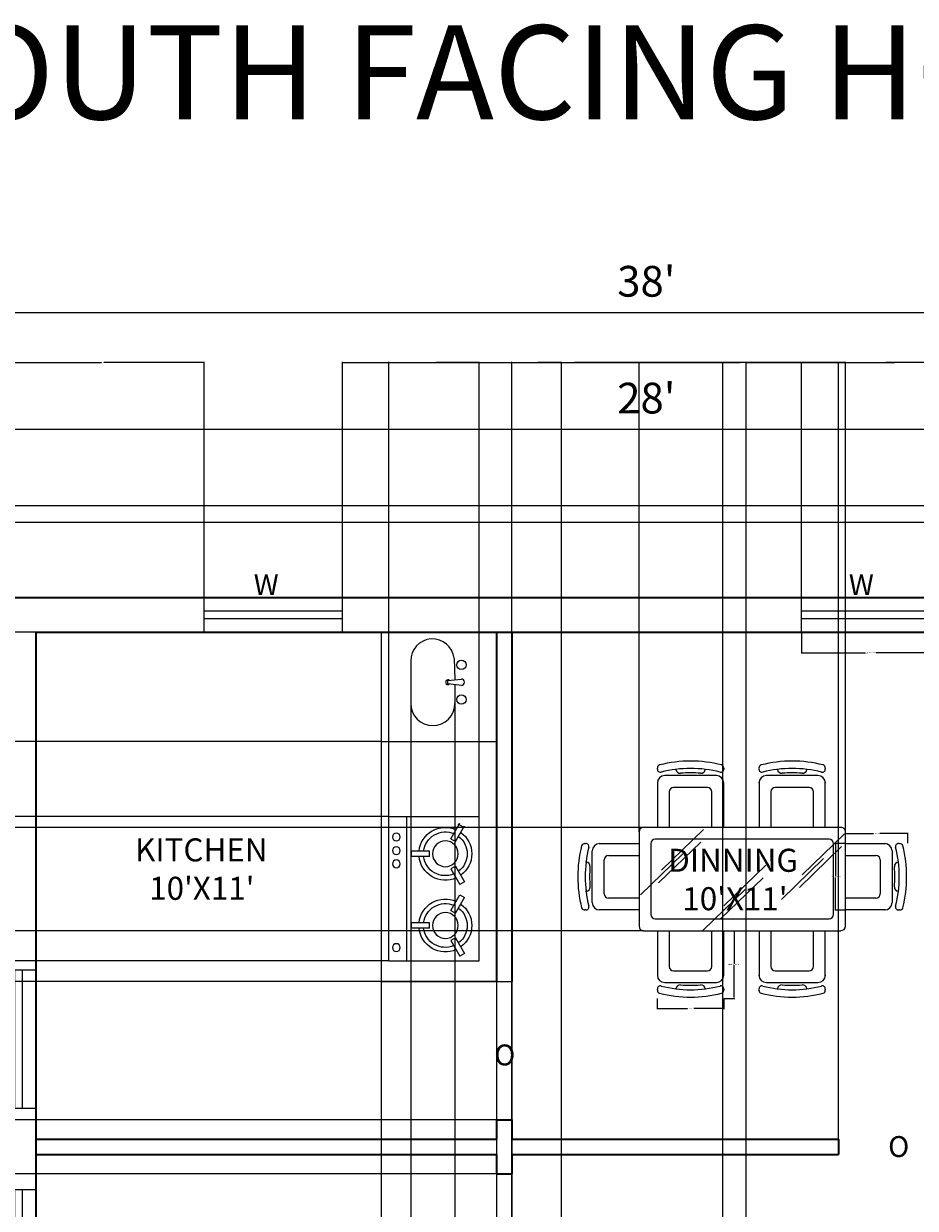
# Model space of a CAD drawing. Units: inches. Extents: x 503 to 1084, y -605 to 132.
# Tile 13 of 14: x 656 to 888, y -177 to 132. Entities that reach past the tile are written whole.
import ezdxf

# ---------------------------------------------------------------- set-up
doc = ezdxf.new("R2010")
doc.units = ezdxf.units.IN
doc.header["$MEASUREMENT"] = 0
for name, color, linetype, lineweight in [('A-ANNO-DIMS', 7, 'Continuous', 18), ('A-ANNO-TEXT', 7, 'Continuous', 18), ('A-AREA-IDEN', 8, 'Continuous', 18), ('A-EQPM', 50, 'Continuous', 18), ('A-FLOR-CASE', 50, 'Continuous', 18), ('A-FLOR-FIXT', 8, 'Continuous', 18), ('C-PROP', 1, 'Continuous', 25), ('wall', 1, 'Continuous', 35), ('wind', 5, 'Continuous', 18)]:
    doc.layers.add(name, color=color, linetype=linetype, lineweight=lineweight)
doc.layers.add('furniture', color=50, linetype='Continuous', lineweight=13, transparency=0.8)
doc.styles.get("Standard").update_dxf_attribs({"font": 'arial.ttf'})
doc.dimstyles.get("Standard").update_dxf_attribs({"dimtxt": 0.18, "dimasz": 0.18, "dimexe": 0.18, "dimexo": 0.0625, "dimgap": 0.09, "dimtad": 0, "dimtih": 1, "dimtoh": 1, "dimdec": 1, "dimzin": 0, "dimdsep": 46, "dimlunit": 4, "dimtxsty": 'Standard', "dimcen": 0.09, "dimadec": 0, "dimazin": 0, "dimtfac": 1, "dimtdec": 1, "dimtofl": 0, "dimtmove": 0, "dimatfit": 3, "dimfxl": 1, "dimtolj": 1, "dimtzin": 0, "dimarcsym": 0})

# ---------------------------------------------------------------- blocks, each defined once
blk = doc.blocks.new('_ArchTick')
at = {"color": 0, "linetype": 'ByBlock', "const_width": 0.15}
blk.add_lwpolyline([(-0.5, -0.5), (0.5, 0.5)], dxfattribs=at)
blk = doc.blocks.new('*D5')
at = {"layer": 'A-ANNO-DIMS', "color": 0, "lineweight": -3, "transparency": 16777216}
blk.add_line((590.09, 56.42), (1046.09, 56.42), dxfattribs=at)
at = {"layer": 'Defpoints', "color": 0, "transparency": 16777216}
for p in [(1046.09, 56.42), (590.09, 6.18), (1046.09, 6.18)]:
    blk.add_point(p, dxfattribs=at)
at = {"layer": 'A-ANNO-DIMS', "color": 0, "lineweight": -3, "transparency": 16777216, "xscale": 5, "yscale": 5, "zscale": 5, "rotation": 180}
blk.add_blockref('_ArchTick', (590.09, 56.42), dxfattribs=at)
at = {"layer": 'A-ANNO-DIMS', "color": 0, "lineweight": -3, "transparency": 16777216, "xscale": 5, "yscale": 5, "zscale": 5}
blk.add_blockref('_ArchTick', (1046.09, 56.42), dxfattribs=at)
at = {"layer": 'A-ANNO-DIMS', "color": 0, "transparency": 16777216, "insert": (818.09, 64.51), "char_height": 8, "attachment_point": 5}
blk.add_mtext("\\A1;38'", dxfattribs=at)
blk = doc.blocks.new('*D7')
at = {"layer": 'A-ANNO-DIMS', "color": 0, "lineweight": -3, "transparency": 16777216}
blk.add_line((650.09, 26.02), (986.09, 26.02), dxfattribs=at)
at = {"layer": 'Defpoints', "color": 0, "transparency": 16777216}
for p in [(986.09, 26.02), (650.09, -17.82), (986.09, -17.82)]:
    blk.add_point(p, dxfattribs=at)
at = {"layer": 'A-ANNO-DIMS', "color": 0, "lineweight": -3, "transparency": 16777216, "xscale": 5, "yscale": 5, "zscale": 5, "rotation": 180}
blk.add_blockref('_ArchTick', (650.09, 26.02), dxfattribs=at)
at = {"layer": 'A-ANNO-DIMS', "color": 0, "lineweight": -3, "transparency": 16777216, "xscale": 5, "yscale": 5, "zscale": 5}
blk.add_blockref('_ArchTick', (986.09, 26.02), dxfattribs=at)
at = {"layer": 'A-ANNO-DIMS', "color": 0, "transparency": 16777216, "insert": (818.09, 34.1), "char_height": 8, "attachment_point": 5}
blk.add_mtext("\\A1;28'", dxfattribs=at)
blk = doc.blocks.new('WIN-36IN')
for p, q in [((0, 0), (0, 9)), ((36, 0), (36, 9)), ((0, 5.5), (36, 5.5)), ((0, 3.5), (36, 3.5))]:
    blk.add_line(p, q)
blk = doc.blocks.new('VENT-24IN')
for p, q in [((0, 9), (0, 0)), ((24, 9), (24, 0)), ((24, 5.5), (0, 5.5)), ((24, 3.5), (0, 3.5))]:
    blk.add_line(p, q)
blk = doc.blocks.new('CHAIR-DINING-END')
for p, q in [((-4.19, -6.72), (-4.19, 6.72)), ((-2.45, 8.63), (-2.05, 8.63)), ((-2.27, 8.63), (7.97, 8.63)), ((-5.82, 3.84), (-5.94, 3.84)), ((-1.12, -4.41), (-1.12, 4.41)), ((0.03, 5.56), (7.97, 5.56)), ((-5.82, -3.84), (-5.94, -3.84)), ((7.97, -5.56), (0.03, -5.56)), ((-2.05, -8.63), (-2.45, -8.63)), ((7.97, -8.63), (-2.27, -8.63))]:
    blk.add_line(p, q)
for centre, radius, start, end in [((24.98, 0), 32.96, 165.853, 194.147), ((-6.23, 7.87), 0.768, 84.0784, 165.853), ((-6.03, 9.78), 1.15, 264.0784, 275.9216), ((24.98, 0), 31.04, 165.6786, 194.3214), ((-5.83, 7.87), 0.768, 345.6786, 95.9216), ((-2.27, 6.72), 1.92, 90, 180), ((-5.94, 2.69), 1.15, 355.0346, 83.9719), ((0.03, 4.41), 1.15, 90, 180), ((24.98, 0), 29.89, 175.0346, 184.9654), ((-5.94, -2.69), 1.15, 276.0281, 4.9654), ((0.03, -4.41), 1.15, 180, 270), ((-6.23, -7.87), 0.768, 194.147, 275.9216), ((-6.03, -9.78), 1.15, 84.0784, 95.9216), ((-5.83, -7.87), 0.768, 264.0784, 14.3214), ((-2.27, -6.72), 1.92, 180, 270)]:
    blk.add_arc(centre, radius, start, end)
blk = doc.blocks.new('CHAIR-DINING-SIDE')
for p, q in [((-3.84, 6.49), (-3.84, 6.61)), ((3.84, 6.49), (3.84, 6.61)), ((-8.63, 3.11), (-8.63, 2.72)), ((6.72, 4.86), (-6.72, 4.86)), ((8.63, 2.72), (8.63, 3.11)), ((-8.63, 2.94), (-8.63, -8.64)), ((-5.56, 0.64), (-5.56, -8.64)), ((4.41, 1.79), (-4.41, 1.79)), ((5.56, -8.64), (5.56, 0.64)), ((8.63, -8.64), (8.63, 2.94))]:
    blk.add_line(p, q)
for centre, radius, start, end in [((-7.87, 6.9), 0.768, 104.147, 185.9216), ((-9.78, 6.7), 1.15, 354.0784, 5.9216), ((-7.87, 6.5), 0.768, 174.0784, 284.3214), ((0, -24.31), 32.96, 75.853, 104.147), ((0, -24.31), 31.04, 75.6786, 104.3214), ((-2.69, 6.61), 1.15, 186.0281, 274.9654), ((2.69, 6.61), 1.15, 265.0346, 353.9719), ((7.87, 6.5), 0.768, 255.6786, 5.9216), ((7.87, 6.9), 0.768, 354.0784, 75.853), ((9.78, 6.7), 1.15, 174.0784, 185.9216), ((-6.72, 2.94), 1.92, 90, 180), ((0, -24.31), 29.89, 85.0346, 94.9654), ((6.72, 2.94), 1.92, 0, 90), ((-4.41, 0.64), 1.15, 90, 180), ((4.41, 0.64), 1.15, 0, 90)]:
    blk.add_arc(centre, radius, start, end)
blk = doc.blocks.new('*D22')
at = {"layer": 'A-ANNO-DIMS', "color": 0, "lineweight": -2, "transparency": 16777216}
for p, q in [((858.5, -26.88), (858.5, -32.4)), ((894.5, -26.88), (894.5, -32.4)), ((858.68, -32.22), (875.12, -32.22)), ((894.32, -32.22), (877.88, -32.22))]:
    blk.add_line(p, q, dxfattribs=at)
at = {"layer": 'A-ANNO-DIMS', "color": 0, "transparency": 16777216}
for points in [[(858.68, -32.19), (858.68, -32.25), (858.5, -32.22)], [(894.32, -32.19), (894.32, -32.25), (894.5, -32.22)]]:
    blk.add_solid(points, dxfattribs=at)
at = {"layer": 'Defpoints', "color": 0, "transparency": 16777216}
for p in [(858.5, -26.82), (894.5, -26.82), (894.5, -32.22)]:
    blk.add_point(p, dxfattribs=at)
at = {"layer": 'A-ANNO-DIMS', "color": 0, "transparency": 16777216, "insert": (876.5, -32.22), "char_height": 0.18, "attachment_point": 5}
blk.add_mtext('\\A1;WINDOW W 3\'-0" TYP.', dxfattribs=at)
blk = doc.blocks.new('*D26')
at = {"layer": 'A-ANNO-DIMS', "color": 0, "lineweight": -2, "transparency": 16777216}
for p, q in [((838.34, -104.56), (841.1, -104.56)), ((840.92, -104.74), (840.92, -113.18)), ((840.92, -121.99), (840.92, -113.55)), ((838.34, -122.17), (841.1, -122.17))]:
    blk.add_line(p, q, dxfattribs=at)
at = {"layer": 'A-ANNO-DIMS', "color": 0, "transparency": 16777216}
for points in [[(840.89, -104.74), (840.95, -104.74), (840.92, -104.56)], [(840.89, -121.99), (840.95, -121.99), (840.92, -122.17)]]:
    blk.add_solid(points, dxfattribs=at)
at = {"layer": 'Defpoints', "color": 0, "transparency": 16777216}
for p in [(838.28, -104.56), (838.28, -122.17), (840.92, -122.17)]:
    blk.add_point(p, dxfattribs=at)
at = {"layer": 'A-ANNO-DIMS', "color": 0, "transparency": 16777216, "insert": (840.92, -113.36), "char_height": 0.18, "attachment_point": 5}
blk.add_mtext('\\A1;SIDE CHAIR 1\'-5 1/2" TYP.', dxfattribs=at)
blk = doc.blocks.new('*D27')
at = {"layer": 'A-ANNO-DIMS', "color": 0, "lineweight": -2, "transparency": 16777216}
for p, q in [((820.94, -122.24), (820.94, -125)), ((838.28, -122.24), (838.28, -125)), ((821.12, -124.82), (828.77, -124.82)), ((838.1, -124.82), (830.45, -124.82))]:
    blk.add_line(p, q, dxfattribs=at)
at = {"layer": 'A-ANNO-DIMS', "color": 0, "transparency": 16777216}
for points in [[(821.12, -124.79), (821.12, -124.85), (820.94, -124.82)], [(838.1, -124.79), (838.1, -124.85), (838.28, -124.82)]]:
    blk.add_solid(points, dxfattribs=at)
at = {"layer": 'Defpoints', "color": 0, "transparency": 16777216}
for p in [(820.94, -122.17), (838.28, -122.17), (820.94, -124.82)]:
    blk.add_point(p, dxfattribs=at)
at = {"layer": 'A-ANNO-DIMS', "color": 0, "transparency": 16777216, "insert": (829.61, -124.82), "char_height": 0.18, "attachment_point": 5}
blk.add_mtext('\\A1;1\'-5 1/2" TYP.', dxfattribs=at)
blk = doc.blocks.new('*D28')
at = {"layer": 'A-ANNO-DIMS', "color": 0, "lineweight": -2, "transparency": 16777216}
for p, q in [((869.85, -81.85), (867.14, -81.85)), ((867.32, -82.03), (867.32, -90.34)), ((867.32, -99.01), (867.32, -90.7)), ((869.85, -99.19), (867.14, -99.19))]:
    blk.add_line(p, q, dxfattribs=at)
at = {"layer": 'A-ANNO-DIMS', "color": 0, "transparency": 16777216}
for points in [[(867.29, -82.03), (867.35, -82.03), (867.32, -81.85)], [(867.29, -99.01), (867.35, -99.01), (867.32, -99.19)]]:
    blk.add_solid(points, dxfattribs=at)
at = {"layer": 'Defpoints', "color": 0, "transparency": 16777216}
for p in [(869.92, -81.85), (867.32, -99.19), (869.92, -99.19)]:
    blk.add_point(p, dxfattribs=at)
at = {"layer": 'A-ANNO-DIMS', "color": 0, "transparency": 16777216, "insert": (867.32, -90.52), "char_height": 0.18, "attachment_point": 5}
blk.add_mtext('\\A1;END CHAIR 1\'-5 1/2" TYP.', dxfattribs=at)
blk = doc.blocks.new('*D29')
at = {"layer": 'A-ANNO-DIMS', "color": 0, "lineweight": -2, "transparency": 16777216}
for p, q in [((869.92, -81.79), (869.92, -79.07)), ((870.1, -79.25), (877.22, -79.25)), ((886.02, -79.25), (878.9, -79.25)), ((886.2, -81.79), (886.2, -79.07))]:
    blk.add_line(p, q, dxfattribs=at)
at = {"layer": 'A-ANNO-DIMS', "color": 0, "transparency": 16777216}
for points in [[(870.1, -79.22), (870.1, -79.28), (869.92, -79.25)], [(886.02, -79.22), (886.02, -79.28), (886.2, -79.25)]]:
    blk.add_solid(points, dxfattribs=at)
at = {"layer": 'Defpoints', "color": 0, "transparency": 16777216}
for p in [(869.92, -79.25), (869.92, -81.85), (886.2, -81.85)]:
    blk.add_point(p, dxfattribs=at)
at = {"layer": 'A-ANNO-DIMS', "color": 0, "transparency": 16777216, "insert": (878.06, -79.25), "char_height": 0.18, "attachment_point": 5}
blk.add_mtext('\\A1;1\'-4 1/2" TYP.', dxfattribs=at)
blk = doc.blocks.new('*D45')
at = {"layer": 'A-ANNO-DIMS', "color": 0, "lineweight": -2, "transparency": 16777216}
for p, q in [((844.09, -354.75), (844.09, 43.51)), ((844.27, 43.33), (879.76, 43.33)), ((915.91, 43.33), (880.42, 43.33)), ((916.09, -354.75), (916.09, 43.51))]:
    blk.add_line(p, q, dxfattribs=at)
at = {"layer": 'A-ANNO-DIMS', "color": 0, "transparency": 16777216}
for points in [[(844.27, 43.36), (844.27, 43.3), (844.09, 43.33)], [(915.91, 43.36), (915.91, 43.3), (916.09, 43.33)]]:
    blk.add_solid(points, dxfattribs=at)
at = {"layer": 'Defpoints', "color": 0, "transparency": 16777216}
for p in [(916.09, 43.33), (844.09, -354.82), (916.09, -354.82)]:
    blk.add_point(p, dxfattribs=at)
at = {"layer": 'A-ANNO-DIMS', "color": 0, "transparency": 16777216, "insert": (880.09, 43.33), "char_height": 0.18, "attachment_point": 5}
blk.add_mtext('\\A1;6\'-0"', dxfattribs=at)
blk = doc.blocks.new('*D46')
at = {"layer": 'A-ANNO-DIMS', "color": 0, "lineweight": -2, "transparency": 16777216}
for p, q in [((796, -354.75), (796, 43.51)), ((796.18, 43.33), (816.67, 43.33)), ((837.82, 43.33), (817.33, 43.33)), ((838, -354.75), (838, 43.51))]:
    blk.add_line(p, q, dxfattribs=at)
at = {"layer": 'A-ANNO-DIMS', "color": 0, "transparency": 16777216}
for points in [[(796.18, 43.36), (796.18, 43.3), (796, 43.33)], [(837.82, 43.36), (837.82, 43.3), (838, 43.33)]]:
    blk.add_solid(points, dxfattribs=at)
at = {"layer": 'Defpoints', "color": 0, "transparency": 16777216}
for p in [(838, 43.33), (796, -354.82), (838, -354.82)]:
    blk.add_point(p, dxfattribs=at)
at = {"layer": 'A-ANNO-DIMS', "color": 0, "transparency": 16777216, "insert": (817, 43.33), "char_height": 0.18, "attachment_point": 5}
blk.add_mtext('\\A1;3\'-6"', dxfattribs=at)
blk = doc.blocks.new('*D48')
at = {"layer": 'A-ANNO-DIMS', "color": 0, "lineweight": -2, "transparency": 16777216}
for p, q in [((783.09, -354.75), (783.09, 43.51)), ((783.27, 43.33), (789.22, 43.33)), ((795.82, 43.33), (789.86, 43.33)), ((796, -354.75), (796, 43.51))]:
    blk.add_line(p, q, dxfattribs=at)
at = {"layer": 'A-ANNO-DIMS', "color": 0, "transparency": 16777216}
for points in [[(783.27, 43.36), (783.27, 43.3), (783.09, 43.33)], [(795.82, 43.36), (795.82, 43.3), (796, 43.33)]]:
    blk.add_solid(points, dxfattribs=at)
at = {"layer": 'Defpoints', "color": 0, "transparency": 16777216}
for p in [(796, 43.33), (783.09, -354.82), (796, -354.82)]:
    blk.add_point(p, dxfattribs=at)
at = {"layer": 'A-ANNO-DIMS', "color": 0, "transparency": 16777216, "insert": (789.54, 43.33), "char_height": 0.18, "attachment_point": 5}
blk.add_mtext('\\A1;1\'-1"', dxfattribs=at)
blk = doc.blocks.new('*D49')
at = {"layer": 'A-ANNO-DIMS', "color": 0, "lineweight": -2, "transparency": 16777216}
for p, q in [((650.09, -17.75), (650.09, 43.51)), ((650.27, 43.33), (676.21, 43.33)), ((702.82, 43.33), (676.88, 43.33)), ((703, -17.75), (703, 43.51))]:
    blk.add_line(p, q, dxfattribs=at)
at = {"layer": 'A-ANNO-DIMS', "color": 0, "transparency": 16777216}
for points in [[(650.27, 43.36), (650.27, 43.3), (650.09, 43.33)], [(702.82, 43.36), (702.82, 43.3), (703, 43.33)]]:
    blk.add_solid(points, dxfattribs=at)
at = {"layer": 'Defpoints', "color": 0, "transparency": 16777216}
for p in [(703, 43.33), (650.09, -17.82), (703, -17.82)]:
    blk.add_point(p, dxfattribs=at)
at = {"layer": 'A-ANNO-DIMS', "color": 0, "transparency": 16777216, "insert": (676.54, 43.33), "char_height": 0.18, "attachment_point": 5}
blk.add_mtext('\\A1;4\'-5"', dxfattribs=at)
blk = doc.blocks.new('*D50')
at = {"layer": 'A-ANNO-DIMS', "color": 0, "lineweight": -2, "transparency": 16777216}
for p, q in [((739, -17.75), (739, 43.51)), ((739.18, 43.33), (798.14, 43.33)), ((858.32, 43.33), (799.36, 43.33)), ((858.5, -17.75), (858.5, 43.51))]:
    blk.add_line(p, q, dxfattribs=at)
at = {"layer": 'A-ANNO-DIMS', "color": 0, "transparency": 16777216}
for points in [[(739.18, 43.36), (739.18, 43.3), (739, 43.33)], [(858.32, 43.36), (858.32, 43.3), (858.5, 43.33)]]:
    blk.add_solid(points, dxfattribs=at)
at = {"layer": 'Defpoints', "color": 0, "transparency": 16777216}
for p in [(858.5, 43.33), (739, -17.82), (858.5, -17.82)]:
    blk.add_point(p, dxfattribs=at)
at = {"layer": 'A-ANNO-DIMS', "color": 0, "transparency": 16777216, "insert": (798.75, 43.33), "char_height": 0.18, "attachment_point": 5}
blk.add_mtext('\\A1;9\'-11 1/2"', dxfattribs=at)
blk = doc.blocks.new('*D56')
at = {"layer": 'A-ANNO-DIMS', "color": 0, "lineweight": -2, "transparency": 16777216}
for p, q in [((779.03, -167.82), (552.76, -167.82)), ((552.94, -168), (552.94, -185.63)), ((552.94, -203.64), (552.94, -186)), ((779.03, -203.82), (552.76, -203.82))]:
    blk.add_line(p, q, dxfattribs=at)
at = {"layer": 'A-ANNO-DIMS', "color": 0, "transparency": 16777216}
for points in [[(552.91, -168), (552.97, -168), (552.94, -167.82)], [(552.91, -203.64), (552.97, -203.64), (552.94, -203.82)]]:
    blk.add_solid(points, dxfattribs=at)
at = {"layer": 'Defpoints', "color": 0, "transparency": 16777216}
for p in [(779.09, -167.82), (552.94, -203.82), (779.09, -203.82)]:
    blk.add_point(p, dxfattribs=at)
at = {"layer": 'A-ANNO-DIMS', "color": 0, "transparency": 16777216, "insert": (552.94, -185.82), "char_height": 0.18, "attachment_point": 5}
blk.add_mtext('\\A1;3\'-0"', dxfattribs=at)
blk = doc.blocks.new('*D57')
at = {"layer": 'A-ANNO-DIMS', "color": 0, "lineweight": -2, "transparency": 16777216}
for p, q in [((868.09, -162.75), (868.09, 43.51)), ((868.27, 43.33), (882.76, 43.33)), ((897.91, 43.33), (883.42, 43.33)), ((898.09, -162.75), (898.09, 43.51))]:
    blk.add_line(p, q, dxfattribs=at)
at = {"layer": 'A-ANNO-DIMS', "color": 0, "transparency": 16777216}
for points in [[(868.27, 43.36), (868.27, 43.3), (868.09, 43.33)], [(897.91, 43.36), (897.91, 43.3), (898.09, 43.33)]]:
    blk.add_solid(points, dxfattribs=at)
at = {"layer": 'Defpoints', "color": 0, "transparency": 16777216}
for p in [(898.09, 43.33), (868.09, -162.82), (898.09, -162.82)]:
    blk.add_point(p, dxfattribs=at)
at = {"layer": 'A-ANNO-DIMS', "color": 0, "transparency": 16777216, "insert": (883.09, 43.33), "char_height": 0.18, "attachment_point": 5}
blk.add_mtext('\\A1;2\'-6"', dxfattribs=at)
blk = doc.blocks.new('*D59')
at = {"layer": 'A-ANNO-DIMS', "color": 0, "lineweight": -2, "transparency": 16777216}
for p, q in [((779.03, -117.82), (552.76, -117.82)), ((552.94, -118), (552.94, -135.63)), ((552.94, -153.64), (552.94, -136)), ((779.03, -153.82), (552.76, -153.82))]:
    blk.add_line(p, q, dxfattribs=at)
at = {"layer": 'A-ANNO-DIMS', "color": 0, "transparency": 16777216}
for points in [[(552.91, -118), (552.97, -118), (552.94, -117.82)], [(552.91, -153.64), (552.97, -153.64), (552.94, -153.82)]]:
    blk.add_solid(points, dxfattribs=at)
at = {"layer": 'Defpoints', "color": 0, "transparency": 16777216}
for p in [(779.09, -117.82), (552.94, -153.82), (779.09, -153.82)]:
    blk.add_point(p, dxfattribs=at)
at = {"layer": 'A-ANNO-DIMS', "color": 0, "transparency": 16777216, "insert": (552.94, -135.82), "char_height": 0.18, "attachment_point": 5}
blk.add_mtext('\\A1;3\'-0"', dxfattribs=at)
blk = doc.blocks.new('*D60')
at = {"layer": 'A-ANNO-DIMS', "color": 0, "lineweight": -2, "transparency": 16777216}
for p, q in [((749.09, -117.88), (749.09, -583.15)), ((779.09, -117.88), (779.09, -583.15)), ((749.27, -582.97), (763.76, -582.97)), ((778.91, -582.97), (764.42, -582.97))]:
    blk.add_line(p, q, dxfattribs=at)
at = {"layer": 'A-ANNO-DIMS', "color": 0, "transparency": 16777216}
for points in [[(749.27, -582.94), (749.27, -583), (749.09, -582.97)], [(778.91, -582.94), (778.91, -583), (779.09, -582.97)]]:
    blk.add_solid(points, dxfattribs=at)
at = {"layer": 'Defpoints', "color": 0, "transparency": 16777216}
for p in [(749.09, -117.82), (779.09, -117.82), (779.09, -582.97)]:
    blk.add_point(p, dxfattribs=at)
at = {"layer": 'A-ANNO-DIMS', "color": 0, "transparency": 16777216, "insert": (764.09, -582.97), "char_height": 0.18, "attachment_point": 5}
blk.add_mtext('\\A1;2\'-6"', dxfattribs=at)
blk = doc.blocks.new('*D61')
at = {"layer": 'A-ANNO-DIMS', "color": 0, "lineweight": -2, "transparency": 16777216}
for p, q in [((749.026202, -26.815853), (552.758702, -26.815853)), ((552.938702, -26.995853), (552.938702, -72.135853)), ((552.938702, -117.635853), (552.938702, -72.495853)), ((749.026202, -117.815853), (552.758702, -117.815853))]:
    blk.add_line(p, q, dxfattribs=at)
at = {"layer": 'A-ANNO-DIMS', "color": 0, "transparency": 16777216}
for points in [[(552.908702, -26.995853), (552.968702, -26.995853), (552.938702, -26.815853)], [(552.908702, -117.635853), (552.968702, -117.635853), (552.938702, -117.815853)]]:
    blk.add_solid(points, dxfattribs=at)
at = {"layer": 'Defpoints', "color": 0, "transparency": 16777216}
for p in [(552.938702, -26.815853), (749.088702, -26.815853), (749.088702, -117.815853)]:
    blk.add_point(p, dxfattribs=at)
at = {"layer": 'A-ANNO-DIMS', "color": 0, "transparency": 16777216, "insert": (552.938702, -72.315853), "char_height": 0.18, "attachment_point": 5}
blk.add_mtext('\\A1;7\'-7"', dxfattribs=at)
blk = doc.blocks.new('*D68')
at = {"layer": 'A-ANNO-DIMS', "color": 0, "lineweight": -2, "transparency": 16777216}
for p, q in [((779.09, -117.88), (779.09, -583.15)), ((783.09, -117.88), (783.09, -583.15)), ((779.27, -582.97), (780.76, -582.97)), ((782.91, -582.97), (781.42, -582.97))]:
    blk.add_line(p, q, dxfattribs=at)
at = {"layer": 'A-ANNO-DIMS', "color": 0, "transparency": 16777216}
for points in [[(779.27, -582.94), (779.27, -583), (779.09, -582.97)], [(782.91, -582.94), (782.91, -583), (783.09, -582.97)]]:
    blk.add_solid(points, dxfattribs=at)
at = {"layer": 'Defpoints', "color": 0, "transparency": 16777216}
for p in [(779.09, -117.82), (783.09, -117.82), (783.09, -582.97)]:
    blk.add_point(p, dxfattribs=at)
at = {"layer": 'A-ANNO-DIMS', "color": 0, "transparency": 16777216, "insert": (781.09, -582.97), "char_height": 0.18, "attachment_point": 5}
blk.add_mtext('\\A1;0\'-4"', dxfattribs=at)
blk = doc.blocks.new('*D69')
at = {"layer": 'A-ANNO-DIMS', "color": 0, "lineweight": -2, "transparency": 16777216}
for p, q in [((816.19, -78.78), (816.19, 43.51)), ((816.37, 43.33), (842.51, 43.33)), ((869.74, 43.33), (843.6, 43.33)), ((869.92, -78.78), (869.92, 43.51))]:
    blk.add_line(p, q, dxfattribs=at)
at = {"layer": 'A-ANNO-DIMS', "color": 0, "transparency": 16777216}
for points in [[(816.37, 43.36), (816.37, 43.3), (816.19, 43.33)], [(869.74, 43.36), (869.74, 43.3), (869.92, 43.33)]]:
    blk.add_solid(points, dxfattribs=at)
at = {"layer": 'Defpoints', "color": 0, "transparency": 16777216}
for p in [(869.92, 43.33), (816.19, -78.84), (869.92, -78.84)]:
    blk.add_point(p, dxfattribs=at)
at = {"layer": 'A-ANNO-DIMS', "color": 0, "transparency": 16777216, "insert": (843.05, 43.33), "char_height": 0.18, "attachment_point": 5}
blk.add_mtext('\\A1;4\'-5 1/2"', dxfattribs=at)
blk = doc.blocks.new('*D70')
at = {"layer": 'A-ANNO-DIMS', "color": 0, "lineweight": -2, "transparency": 16777216}
for p, q in [((817.28, -77.69), (552.76, -77.69)), ((552.94, -77.87), (552.94, -90.94)), ((552.94, -104.38), (552.94, -91.31)), ((817.28, -104.56), (552.76, -104.56))]:
    blk.add_line(p, q, dxfattribs=at)
at = {"layer": 'A-ANNO-DIMS', "color": 0, "transparency": 16777216}
for points in [[(552.91, -77.87), (552.97, -77.87), (552.94, -77.69)], [(552.91, -104.38), (552.97, -104.38), (552.94, -104.56)]]:
    blk.add_solid(points, dxfattribs=at)
at = {"layer": 'Defpoints', "color": 0, "transparency": 16777216}
for p in [(817.34, -77.69), (552.94, -104.56), (817.34, -104.56)]:
    blk.add_point(p, dxfattribs=at)
at = {"layer": 'A-ANNO-DIMS', "color": 0, "transparency": 16777216, "insert": (552.94, -91.12), "char_height": 0.18, "attachment_point": 5}
blk.add_mtext('\\A1;2\'-3"', dxfattribs=at)
blk = doc.blocks.new('*D73')
at = {"layer": 'A-ANNO-DIMS', "color": 0, "lineweight": -2, "transparency": 16777216}
for p, q in [((751.07, -74.77), (751.07, 43.51)), ((751.25, 43.33), (762.21, 43.33)), ((774.37, 43.33), (763.41, 43.33)), ((774.55, -74.77), (774.55, 43.51))]:
    blk.add_line(p, q, dxfattribs=at)
at = {"layer": 'A-ANNO-DIMS', "color": 0, "transparency": 16777216}
for points in [[(751.25, 43.36), (751.25, 43.3), (751.07, 43.33)], [(774.37, 43.36), (774.37, 43.3), (774.55, 43.33)]]:
    blk.add_solid(points, dxfattribs=at)
at = {"layer": 'Defpoints', "color": 0, "transparency": 16777216}
for p in [(774.55, 43.33), (751.07, -74.83), (774.55, -74.83)]:
    blk.add_point(p, dxfattribs=at)
at = {"layer": 'A-ANNO-DIMS', "color": 0, "transparency": 16777216, "insert": (762.81, 43.33), "char_height": 0.18, "attachment_point": 5}
blk.add_mtext('\\A1;1\'-11 1/2"', dxfattribs=at)
blk = doc.blocks.new('*D74')
at = {"layer": 'A-ANNO-DIMS', "color": 0, "lineweight": -2, "transparency": 16777216}
for p, q in [((751.01, -74.83), (552.76, -74.83)), ((552.94, -75.01), (552.94, -93.43)), ((552.94, -112.21), (552.94, -93.8)), ((751.01, -112.39), (552.76, -112.39))]:
    blk.add_line(p, q, dxfattribs=at)
at = {"layer": 'A-ANNO-DIMS', "color": 0, "transparency": 16777216}
for points in [[(552.91, -75.01), (552.97, -75.01), (552.94, -74.83)], [(552.91, -112.21), (552.97, -112.21), (552.94, -112.39)]]:
    blk.add_solid(points, dxfattribs=at)
at = {"layer": 'Defpoints', "color": 0, "transparency": 16777216}
for p in [(751.07, -74.83), (552.94, -112.39), (751.07, -112.39)]:
    blk.add_point(p, dxfattribs=at)
at = {"layer": 'A-ANNO-DIMS', "color": 0, "transparency": 16777216, "insert": (552.94, -93.61), "char_height": 0.18, "attachment_point": 5}
blk.add_mtext('\\A1;3\'-1 1/2"', dxfattribs=at)
blk = doc.blocks.new('*D75')
at = {"layer": 'A-ANNO-DIMS', "color": 0, "lineweight": -2, "transparency": 16777216}
for p, q in [((749.03, -26.82), (552.76, -26.82)), ((552.94, -27), (552.94, -40.85)), ((552.94, -55.08), (552.94, -41.22)), ((749.03, -55.26), (552.76, -55.26))]:
    blk.add_line(p, q, dxfattribs=at)
at = {"layer": 'A-ANNO-DIMS', "color": 0, "transparency": 16777216}
for points in [[(552.91, -27), (552.97, -27), (552.94, -26.82)], [(552.91, -55.08), (552.97, -55.08), (552.94, -55.26)]]:
    blk.add_solid(points, dxfattribs=at)
at = {"layer": 'Defpoints', "color": 0, "transparency": 16777216}
for p in [(749.09, -26.82), (552.94, -55.26), (749.09, -55.26)]:
    blk.add_point(p, dxfattribs=at)
at = {"layer": 'A-ANNO-DIMS', "color": 0, "transparency": 16777216, "insert": (552.94, -41.04), "char_height": 0.18, "attachment_point": 5}
blk.add_mtext('\\A1;2\'-4 1/2"', dxfattribs=at)
blk = doc.blocks.new('*D76')
at = {"layer": 'A-ANNO-DIMS', "color": 0, "lineweight": -2, "transparency": 16777216}
for p, q in [((756.77, -45.47), (756.77, -583.15)), ((768.24, -45.47), (768.24, -583.15)), ((756.95, -582.97), (761.9, -582.97)), ((768.06, -582.97), (763.11, -582.97))]:
    blk.add_line(p, q, dxfattribs=at)
at = {"layer": 'A-ANNO-DIMS', "color": 0, "transparency": 16777216}
for points in [[(756.95, -582.94), (756.95, -583), (756.77, -582.97)], [(768.06, -582.94), (768.06, -583), (768.24, -582.97)]]:
    blk.add_solid(points, dxfattribs=at)
at = {"layer": 'Defpoints', "color": 0, "transparency": 16777216}
for p in [(756.77, -45.4), (768.24, -45.4), (768.24, -582.97)]:
    blk.add_point(p, dxfattribs=at)
at = {"layer": 'A-ANNO-DIMS', "color": 0, "transparency": 16777216, "insert": (762.51, -582.97), "char_height": 0.18, "attachment_point": 5}
blk.add_mtext('\\A1;0\'-11 1/2"', dxfattribs=at)

msp = doc.modelspace()

# ---------------------------------------------------------------- linework, layer by layer
at = {"layer": 'A-EQPM'}
for p, q in [((751.07, -112.39), (751.07, -74.83)), ((751.07, -74.83), (774.55, -74.83)), ((755.77, -112.39), (755.77, -74.83)), ((767.21, -80.63), (769.55, -76.58)), ((769, -76.77), (770.36, -77.55)), ((774.55, -112.39), (774.55, -74.83)), ((768.43, -81.33), (770.77, -77.28)), ((767.21, -80.63), (768.43, -81.33)), ((761.65, -83.83), (756.98, -83.83)), ((756.98, -85.24), (756.98, -83.83)), ((761.65, -85.24), (756.98, -85.24)), ((761.65, -85.24), (761.65, -83.83)), ((768.43, -87.75), (767.21, -88.45)), ((767.21, -88.45), (769.54, -92.5)), ((768.43, -87.75), (770.76, -91.8)), ((770.76, -91.8), (769.54, -92.5)), ((767.21, -99.29), (769.55, -95.24)), ((769.55, -95.24), (770.77, -95.95)), ((768.43, -100), (770.77, -95.95)), ((767.21, -99.29), (768.43, -100)), ((761.65, -102.5), (756.98, -102.5)), ((756.98, -103.9), (756.98, -102.5)), ((761.65, -103.91), (756.98, -103.9)), ((761.65, -103.91), (761.65, -102.5)), ((768.43, -106.41), (767.21, -107.11)), ((767.21, -107.11), (769.54, -111.17)), ((768.43, -106.41), (770.76, -110.46)), ((770.76, -110.46), (769.54, -111.17)), ((751.07, -112.39), (774.55, -112.39))]:
    msp.add_line(p, q, dxfattribs=at)
at = {"layer": 'A-EQPM', "extrusion": (0, 0, -1)}
for centre, major_axis, start_param, end_param in [((753, -80.18), (0.72, 0.72), 2.35619449019219, 8.639379797371777), ((765.76, -84.54), (6.88, 0), 3.2451, 5.134376), ((765.76, -84.54), (4.03, 4.03), 4.051123, 5.898002), ((765.76, -84.54), (4.03, 4.03), 6.145519, 7.992397), ((765.76, -84.54), (6.88, 0.01), -0.942584, 0.946692), ((753, -83.71), (0.72, 0.72), 2.35619449019219, 8.639379797371777), ((765.76, -84.54), (2.37, 2.37), 2.356194490192312, 8.639379797371898), ((753, -87.16), (0.72, 0.72), 2.35619449019219, 8.639379797371777), ((765.76, -84.54), (6.88, -0.01), 1.148752, 3.038029), ((765.76, -84.54), (4.03, -4.03), 0.385932, 2.23281), ((765.76, -103.2), (6.88, 0), 3.244173, 5.13345), ((765.76, -103.2), (4.03, -4.03), 2.480327, 4.327205), ((765.76, -103.2), (4.03, 4.03), 6.145519, 7.992397), ((765.76, -103.2), (6.88, 0), -0.944011, 0.945266), ((765.76, -103.2), (2.37, 2.37), 2.356194490192306, 8.639379797371893), ((765.76, -103.2), (6.88, -0.01), 1.14879, 3.038067), ((765.76, -103.2), (4.03, -4.03), 0.385932, 2.23281), ((753, -108.96), (0.72, 0.72), 2.35619449019219, 8.639379797371777)]:
    msp.add_ellipse(centre, major_axis=major_axis, ratio=1, start_param=start_param, end_param=end_param, dxfattribs=at)
at = {"layer": 'A-FLOR-CASE'}
for p, q in [((749.09, -26.82), (749.09, -117.82)), ((749.09, -55.26), (779.13, -55.26)), ((749.09, -117.82), (783.09, -117.82))]:
    msp.add_line(p, q, dxfattribs=at)
at = {"layer": 'A-FLOR-FIXT'}
for p, q in [((768.04, -33.62), (768.2, -39.25)), ((756.77, -34.34), (756.77, -45.4)), ((766.45, -39.46), (769.94, -39.05)), ((766.45, -40.34), (766.45, -39.46)), ((769.94, -40.69), (766.45, -40.28)), ((768.24, -40.49), (768.24, -45.4))]:
    msp.add_line(p, q, dxfattribs=at)
for centre in [(769.94, -35.36), (769.94, -44.38)]:
    msp.add_circle(centre, 1.23, dxfattribs=at)
for centre, radius, start, end in [((762.42, -34.25), 5.65, 6.3659, 180.8792), ((766.45, -39.87), 0.615, 48.1701, 311.8299), ((769.94, -39.87), 0.82, 270, 90), ((762.51, -45.4), 5.74, 180, 0)]:
    msp.add_arc(centre, radius, start, end, dxfattribs=at)
at = {"layer": 'C-PROP'}
for p, q in [((590.09, 6.18), (1046.09, 6.18)), ((1041.59, 1.68), (594.59, 1.68))]:
    msp.add_line(p, q, dxfattribs=at)
at = {"layer": 'furniture'}
for p, q in [((816.19, -78.84), (816.19, -103.4)), ((868.76, -77.69), (817.34, -77.69)), ((833.01, -78.19), (822.03, -88.82)), ((869.67, -79.37), (858.69, -90)), ((869.92, -103.4), (869.92, -78.84)), ((819.26, -81.91), (819.26, -100.33)), ((865.69, -80.76), (820.41, -80.76)), ((832.25, -81.5), (821.27, -92.14)), ((868.91, -82.68), (857.93, -93.32)), ((866.85, -100.33), (866.85, -81.91)), ((827.58, -84.59), (816.59, -95.22)), ((864.23, -85.77), (853.25, -96.41)), ((849.23, -87.47), (838.25, -98.1)), ((848.47, -90.79), (837.48, -101.42)), ((843.79, -93.87), (832.81, -104.51)), ((820.41, -101.49), (865.69, -101.49)), ((817.34, -104.56), (868.76, -104.56))]:
    msp.add_line(p, q, dxfattribs=at)
for centre, radius, start, end in [((817.34, -78.84), 1.15, 90, 180), ((868.82, -78.79), 1.1, 357.166, 92.834), ((820.41, -81.91), 1.15, 90, 180), ((865.69, -81.91), 1.15, 0, 90), ((820.41, -100.33), 1.15, 180, 270), ((865.69, -100.33), 1.15, 270, 0), ((817.34, -103.4), 1.15, 180, 270), ((868.76, -103.4), 1.15, 270, 0)]:
    msp.add_arc(centre, radius, start, end, dxfattribs=at)
at = {"layer": 'wall'}
for p, q in [((650.09, -17.82), (986.09, -17.82)), ((659.09, -26.82), (977.09, -26.82)), ((659.09, -26.82), (659.09, -433.82)), ((779.09, -26.82), (779.09, -117.82)), ((783.09, -26.82), (783.09, -117.82)), ((779.09, -153.82), (783.09, -153.82)), ((779.09, -153.82), (779.09, -158.82)), ((783.09, -153.82), (783.09, -158.82)), ((659.09, -158.82), (779.09, -158.82)), ((783.09, -158.82), (868.09, -158.82)), ((868.09, -158.82), (868.09, -162.82)), ((659.09, -162.82), (779.09, -162.82)), ((779.09, -162.82), (779.09, -167.82)), ((783.09, -162.82), (868.09, -162.82)), ((783.09, -162.82), (783.09, -167.82)), ((779.09, -167.82), (783.09, -167.82))]:
    msp.add_line(p, q, dxfattribs=at)

# ---------------------------------------------------------------- block references
at = {"layer": 'furniture'}
for name, p in [('CHAIR-DINING-SIDE', (829.61, -69.05)), ('CHAIR-DINING-SIDE', (856.06, -69.05)), ('CHAIR-DINING-END', (808.22, -90.52))]:
    msp.add_blockref(name, p, dxfattribs=at)
at = {"layer": 'furniture', "rotation": 180}
for name, p in [('CHAIR-DINING-END', (877.89, -90.52)), ('CHAIR-DINING-SIDE', (829.61, -113.2)), ('CHAIR-DINING-SIDE', (856.06, -113.2))]:
    msp.add_blockref(name, p, dxfattribs=at)
at = {"layer": 'wind'}
for p in [(703, -26.82), (858.51, -26.82)]:
    msp.add_blockref('WIN-36IN', p, dxfattribs=at)
for name, p, rotation in [('WIN-36IN', (650.08, -114.78), 270), ('VENT-24IN', (659.09, -195.98), 90.00000000000081)]:
    msp.add_blockref(name, p, dxfattribs=dict(at, rotation=rotation))

# ---------------------------------------------------------------- texts
at = {"layer": 'A-ANNO-TEXT'}
for s, p in [('W', (715.86, -17.2)), ('W', (870.81, -17.2)), ('O', (778.47, -139.63)), ('O', (881.05, -163.48))]:
    msp.add_text(s, height=5.44, dxfattribs=at).set_placement(p)
at = {"layer": 'A-ANNO-TEXT', "insert": (619.28, 131.14), "char_height": 24.4528, "attachment_point": 1}
msp.add_mtext_dynamic_manual_height_columns('SOUTH FACING HOUSE', width=395.3147, gutter_width=4.08, heights=[0], dxfattribs=at)
at = {"layer": 'A-AREA-IDEN', "char_height": 6, "attachment_point": 1}
for s, width, insert in [("    KITCHEN\\P      10'X11'", 54.3765, (677.64, -80.52)), ("    DINNING\\P      10'X11'", 53.3957, (816.45, -83.23))]:
    msp.add_mtext_dynamic_manual_height_columns(s, width=width, gutter_width=1, heights=[0], dxfattribs=dict(at, insert=insert))

# ---------------------------------------------------------------- dimensions: what is measured, and where the dimension line sits
at = {"layer": 'A-ANNO-DIMS'}
for base, p1, p2, override, picture, middle in [((1046.09, 56.42), (590.09, 6.18), (1046.09, 6.18), {"dimtxt": 8, "dimasz": 5, "dimgap": 4, "dimtad": 1, "dimblk1": 'ArchTick', "dimblk2": 'ArchTick', "dimsah": 1, "dimse1": 1, "dimse2": 1, "dimclrd": 0, "dimclre": 0, "dimclrt": 0, "dimlwd": -3}, '*D5', (818.09, 64.51)), ((703, 43.33), (650.09, -17.82), (703, -17.82), {"dimdec": 1, "dimlfac": 1, "dimrnd": 0, "dimzin": 1, "dimdsep": 46, "dimlunit": 4, "dimfrac": 2}, '*D49', (676.54, 43.33)), ((858.5, 43.33), (739, -17.82), (858.5, -17.82), {"dimdec": 1, "dimlfac": 1, "dimrnd": 0, "dimzin": 1, "dimdsep": 46, "dimlunit": 4, "dimfrac": 2}, '*D50', (798.75, 43.33)), ((774.55, 43.33), (751.07, -74.83), (774.55, -74.83), {"dimdec": 1, "dimlfac": 1, "dimrnd": 0, "dimzin": 1, "dimdsep": 46, "dimlunit": 4, "dimfrac": 2}, '*D73', (762.81, 43.33)), ((796, 43.33), (783.09, -354.82), (796, -354.82), {"dimdec": 1, "dimlfac": 1, "dimrnd": 0, "dimzin": 1, "dimdsep": 46, "dimlunit": 4, "dimfrac": 2}, '*D48', (789.54, 43.33)), ((838, 43.33), (796, -354.82), (838, -354.82), {"dimdec": 1, "dimlfac": 1, "dimrnd": 0, "dimzin": 1, "dimdsep": 46, "dimlunit": 4, "dimfrac": 2}, '*D46', (817, 43.33)), ((869.92, 43.33), (816.19, -78.84), (869.92, -78.84), {"dimdec": 1, "dimlfac": 1, "dimrnd": 0, "dimzin": 1, "dimdsep": 46, "dimlunit": 4, "dimfrac": 2}, '*D69', (843.05, 43.33)), ((916.09, 43.33), (844.09, -354.82), (916.09, -354.82), {"dimdec": 1, "dimlfac": 1, "dimrnd": 0, "dimzin": 1, "dimdsep": 46, "dimlunit": 4, "dimfrac": 2}, '*D45', (880.09, 43.33)), ((898.09, 43.33), (868.09, -162.82), (898.09, -162.82), {"dimdec": 1, "dimlfac": 1, "dimrnd": 0, "dimzin": 1, "dimdsep": 46, "dimlunit": 4, "dimfrac": 2}, '*D57', (883.09, 43.33)), ((986.09, 26.02), (650.09, -17.82), (986.09, -17.82), {"dimtxt": 8, "dimasz": 5, "dimgap": 4, "dimtad": 1, "dimblk1": 'ArchTick', "dimblk2": 'ArchTick', "dimsah": 1, "dimse1": 1, "dimse2": 1, "dimclrd": 0, "dimclre": 0, "dimclrt": 0, "dimlwd": -3}, '*D7', (818.09, 34.1)), ((768.24, -582.97), (756.77, -45.4), (768.24, -45.4), {"dimdec": 1, "dimlfac": 1, "dimrnd": 0, "dimzin": 1, "dimdsep": 46, "dimlunit": 4, "dimfrac": 2}, '*D76', (762.51, -582.97)), ((779.09, -582.97), (749.09, -117.82), (779.09, -117.82), {"dimdec": 1, "dimlfac": 1, "dimrnd": 0, "dimzin": 1, "dimdsep": 46, "dimlunit": 4, "dimfrac": 2}, '*D60', (764.09, -582.97)), ((783.09, -582.97), (779.09, -117.82), (783.09, -117.82), {"dimdec": 1, "dimlfac": 1, "dimrnd": 0, "dimzin": 1, "dimdsep": 46, "dimlunit": 4, "dimfrac": 2}, '*D68', (781.09, -582.97))]:
    dim = msp.add_linear_dim(base=base, p1=p1, p2=p2, dimstyle='Standard', override=override, dxfattribs=at)
    dim.commit()
    dim.dimension.update_dxf_attribs({"geometry": picture, "text_midpoint": middle})
for base, p1, p2, picture, middle in [((552.94, -55.26), (749.09, -26.82), (749.09, -55.26), '*D75', (552.94, -41.04)), ((552.94, -26.82), (749.09, -117.82), (749.09, -26.82), '*D61', (552.94, -72.32)), ((552.94, -112.39), (751.07, -74.83), (751.07, -112.39), '*D74', (552.94, -93.61)), ((552.94, -104.56), (817.34, -77.69), (817.34, -104.56), '*D70', (552.94, -91.12)), ((552.94, -153.82), (779.09, -117.82), (779.09, -153.82), '*D59', (552.94, -135.82)), ((552.94, -203.82), (779.09, -167.82), (779.09, -203.82), '*D56', (552.94, -185.82))]:
    dim = msp.add_linear_dim(base=base, p1=p1, p2=p2, angle=90, dimstyle='Standard', override={"dimdec": 1, "dimlfac": 1, "dimrnd": 0, "dimzin": 1, "dimdsep": 46, "dimlunit": 4, "dimfrac": 2}, dxfattribs=at)
    dim.commit()
    dim.dimension.update_dxf_attribs({"geometry": picture, "text_midpoint": middle})
dim = msp.add_linear_dim(base=(894.5, -32.22), p1=(858.5, -26.82), p2=(894.5, -26.82), text='WINDOW W <> TYP.', dimstyle='Standard', override={"dimdec": 1, "dimlfac": 1, "dimrnd": 0, "dimzin": 1, "dimdsep": 46, "dimlunit": 4, "dimfrac": 2}, dxfattribs=at)
dim.commit()
dim.dimension.update_dxf_attribs({"geometry": '*D22', "text_midpoint": (876.5, -32.22)})
for base, p1, p2, angle, text, picture, middle in [((869.92, -79.25), (886.2, -81.85), (869.92, -81.85), 180, '<> TYP.', '*D29', (878.06, -79.25)), ((867.32, -99.19), (869.92, -81.85), (869.92, -99.19), 270, 'END CHAIR <> TYP.', '*D28', (867.32, -90.52)), ((840.92, -122.17), (838.28, -104.56), (838.28, -122.17), 270, 'SIDE CHAIR <> TYP.', '*D26', (840.92, -113.36)), ((820.94, -124.82), (838.28, -122.17), (820.94, -122.17), 180, '<> TYP.', '*D27', (829.61, -124.82))]:
    dim = msp.add_linear_dim(base=base, p1=p1, p2=p2, angle=angle, text=text, dimstyle='Standard', override={"dimdec": 1, "dimlfac": 1, "dimrnd": 0, "dimzin": 1, "dimdsep": 46, "dimlunit": 4, "dimfrac": 2}, dxfattribs=at)
    dim.commit()
    dim.dimension.update_dxf_attribs({"geometry": picture, "text_midpoint": middle})

doc.saveas('drawing.dxf')
